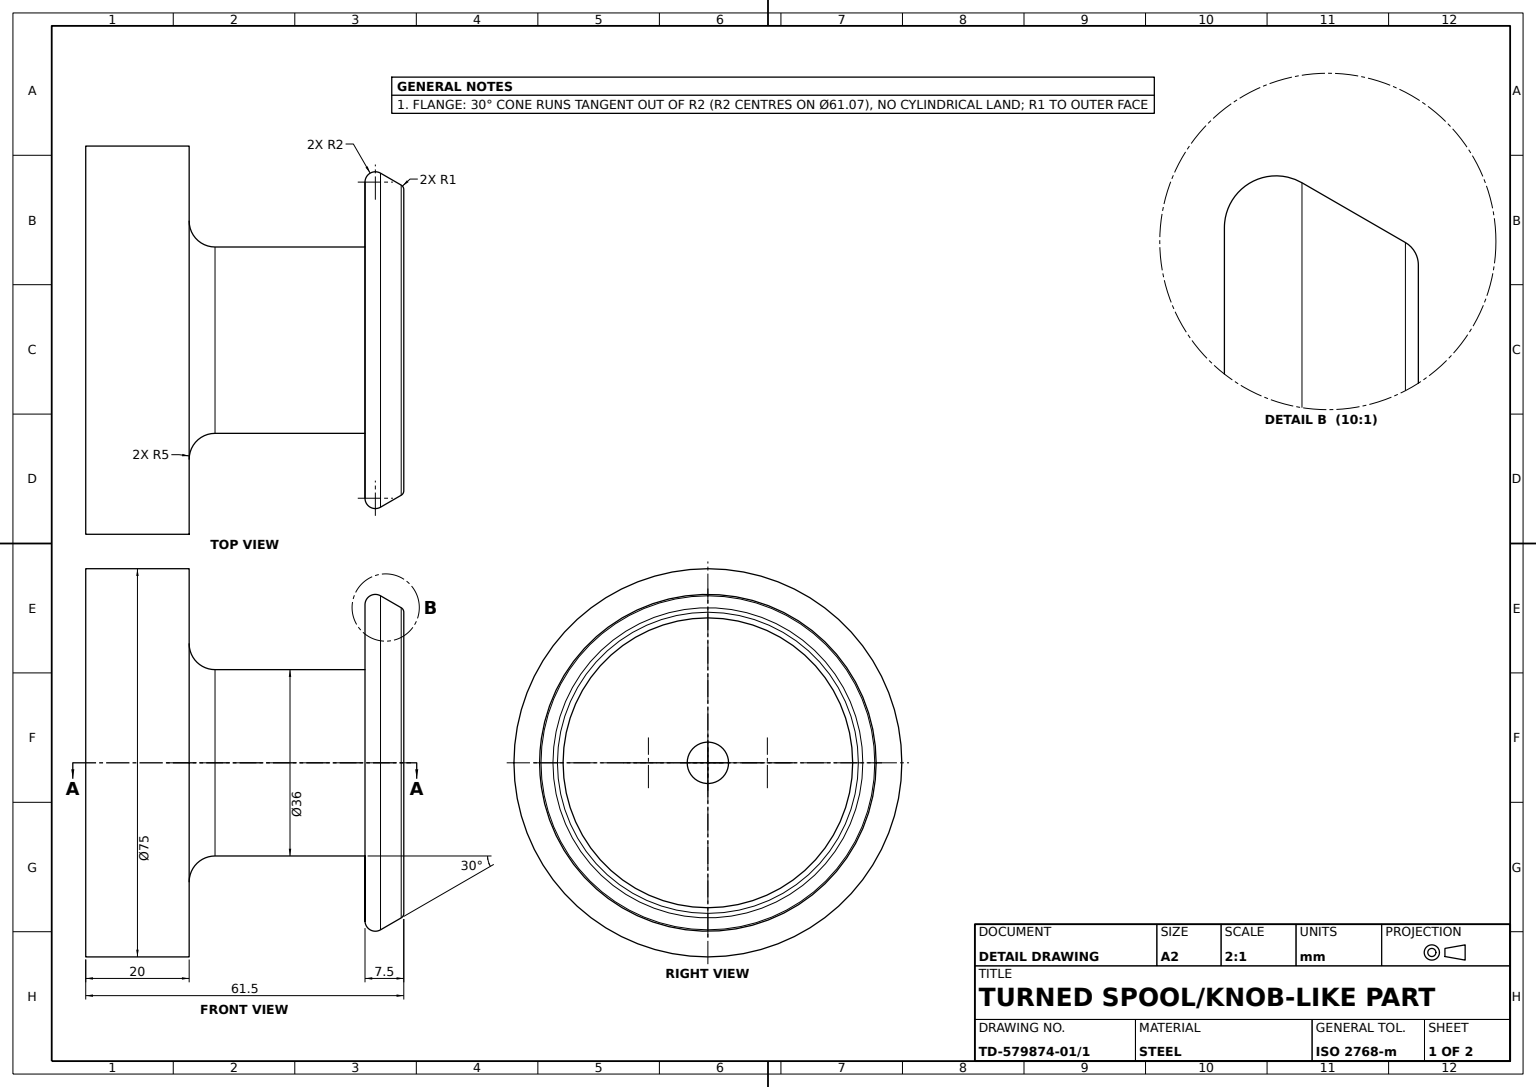
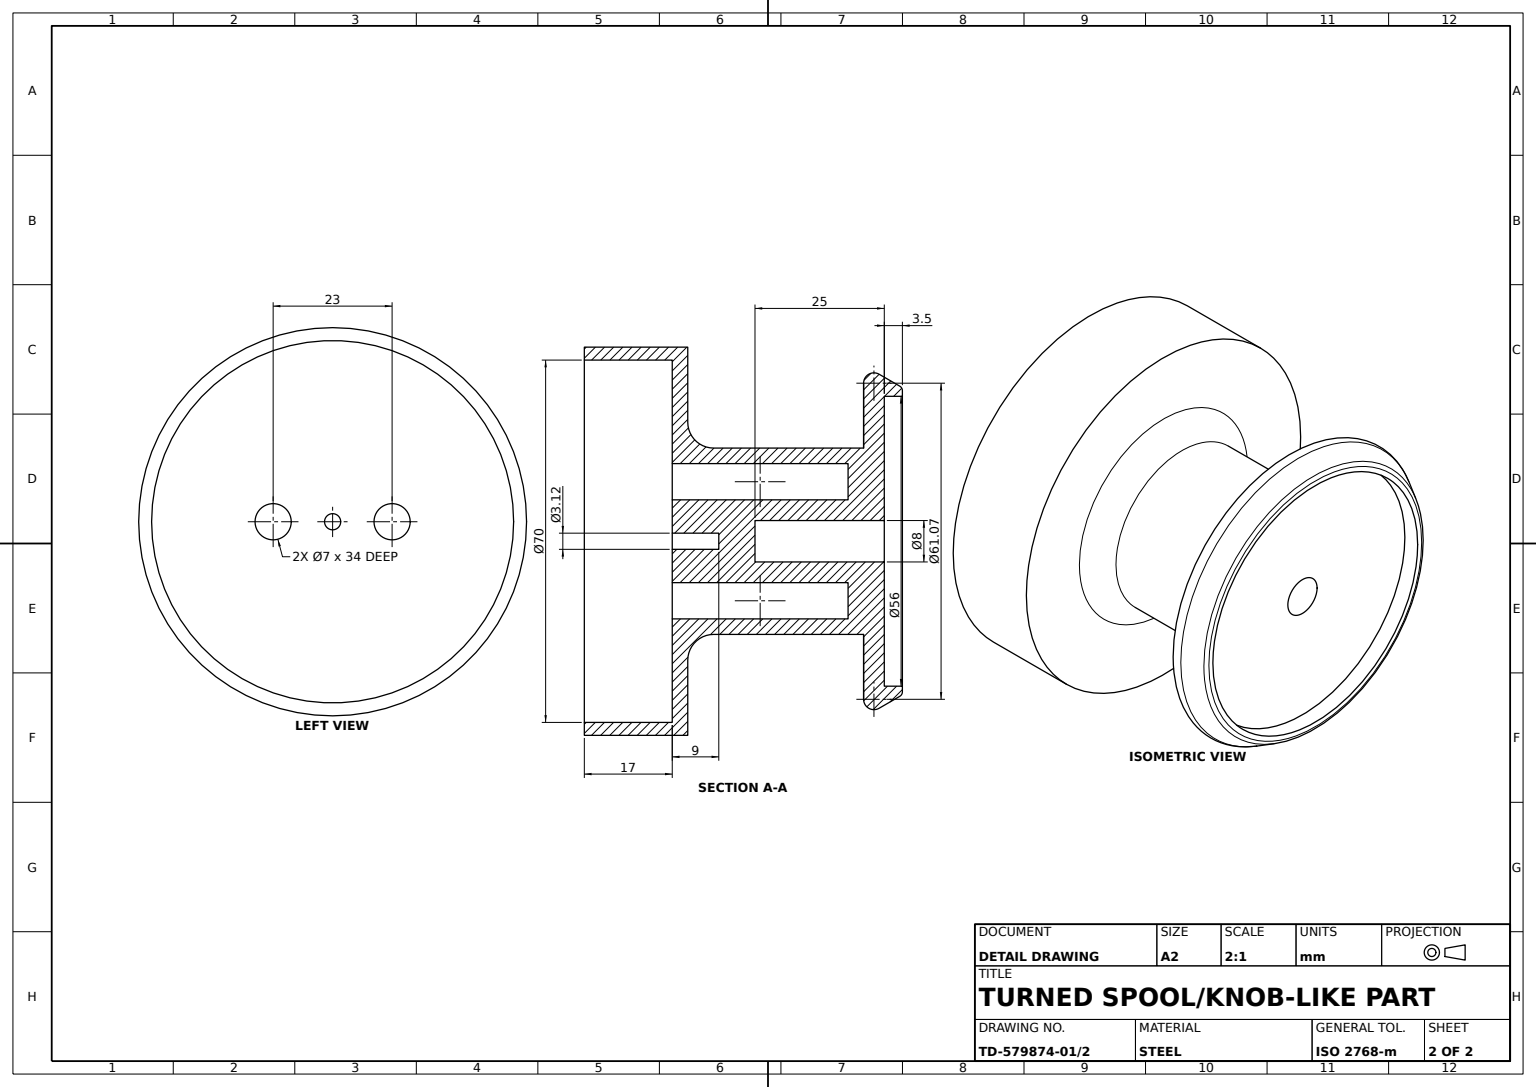
from build123d import *

# Parameters (mm, degrees)
BASE_DISC_SKETCH_75_R        = 37.5
BASE_DISC_75_DEPTH           = 20
NECK_SKETCH_36_R             = 18
NECK_36_DEPTH                = 34
NECK_ROOT_FILLET_R5_R        = 5
TOP_FLANGE_SKETCH_68_R       = 34
TOP_FLANGE_68_DRAFTED_DEPTH  = 7.5
TOP_FLANGE_68_DRAFTED_TAPER  = 30
TOP_RECESS_SKETCH_56_R       = 28
TOP_RECESS_56_DEPTH          = 3.5
FLANGE_EDGE_FILLET_R1_R      = 1
FLANGE_EDGE_FILLET_R2_R      = 2
BASE_RECESS_SKETCH_70_R      = 35
BASE_RECESS_70_DEPTH         = 17
BASE_POCKET_PROFILE_SKETCH_R = 3.5
BASE_POCKET_CUT_34MM_DEPTH   = 34
SKETCH32_4_R                 = 1.562112032
BASE_POCKET_CUT_9MM_DEPTH    = 9
CENTRE_HOLE_SKETCH_8_R       = 4
CENTRE_HOLE_8_DEPTH          = 25


with BuildPart() as part:
    # Base Disc Sketch _75 → Base Disc _75 (new body)
    with BuildSketch(Plane(origin=(0, 0, 0), x_dir=(1, 0, 0), z_dir=(0, 1, 0))):
        with Locations(Location((0, 0, 0), (0, 0, 270))):
            Circle(BASE_DISC_SKETCH_75_R)
    extrude(amount=BASE_DISC_75_DEPTH)

    # Neck Sketch _36 → Neck _36 (add)
    with BuildSketch(Plane(origin=(0, 20, 0), x_dir=(1, 0, 0), z_dir=(0, 1, 0))):
        with Locations(Location((0, 0, 0), (0, 0, 270))):
            Circle(NECK_SKETCH_36_R)
    extrude(amount=NECK_36_DEPTH)

    # Neck Root Fillet R5
    neck_root_fillet_r5_edges = [part.edges().sort_by_distance(p)[0] for p in [
        (0, 20, -18),
    ]]
    fillet(neck_root_fillet_r5_edges, radius=NECK_ROOT_FILLET_R5_R)

    # Top Flange Sketch _68 → Top Flange _68 Drafted (add)
    with BuildSketch(Plane(origin=(0, 54, 0), x_dir=(1, 0, 0), z_dir=(0, 1, 0))):
        Circle(TOP_FLANGE_SKETCH_68_R)
    extrude(amount=TOP_FLANGE_68_DRAFTED_DEPTH, taper=TOP_FLANGE_68_DRAFTED_TAPER)

    # Top Recess Sketch _56 → Top Recess _56 (cut)
    with BuildSketch(Plane(origin=(0, 61.5, 0), x_dir=(1, 0, 0), z_dir=(0, 1, 0))):
        with Locations(Location((0, 0, 0), (0, 0, 270))):
            Circle(TOP_RECESS_SKETCH_56_R)
    extrude(amount=-TOP_RECESS_56_DEPTH, mode=Mode.SUBTRACT)

    # Flange Edge Fillet R1
    flange_edge_fillet_r1_edges = [part.edges().sort_by_distance(p)[0] for p in [
        (-29.669872981, 61.5, 0),
    ]]
    fillet(flange_edge_fillet_r1_edges, radius=FLANGE_EDGE_FILLET_R1_R)

    # Flange Edge Fillet R2
    flange_edge_fillet_r2_edges = [part.edges().sort_by_distance(p)[0] for p in [
        (-34, 54, 0),
    ]]
    fillet(flange_edge_fillet_r2_edges, radius=FLANGE_EDGE_FILLET_R2_R)

    # Base Recess Sketch _70 → Base Recess _70 (cut)
    with BuildSketch(Plane.XZ):
        with Locations(Location((0, 0, 0), (0, 0, 270))):
            Circle(BASE_RECESS_SKETCH_70_R)
    extrude(amount=-BASE_RECESS_70_DEPTH, mode=Mode.SUBTRACT)

    # Base Pocket Profile Sketch → Base Pocket Cut 34mm (cut)
    with BuildSketch(Plane.XZ.offset(-17)):
        with Locations(Location((0, -11.5, 0), (0, 0, 270))):
            Circle(BASE_POCKET_PROFILE_SKETCH_R)
        with Locations(Location((0, 11.5, 0), (0, 0, 270))):
            Circle(BASE_POCKET_PROFILE_SKETCH_R)
    extrude(amount=-BASE_POCKET_CUT_34MM_DEPTH, mode=Mode.SUBTRACT)

    # Sketch32_4 → Base Pocket Cut 9mm (cut)
    with BuildSketch(Plane.XZ.offset(-17)):
        with Locations(Location((0, 0, 0), (0, 0, 270))):
            Circle(SKETCH32_4_R)
    extrude(amount=-BASE_POCKET_CUT_9MM_DEPTH, mode=Mode.SUBTRACT)

    # Centre Hole Sketch _8 → Centre Hole _8 (cut)
    with BuildSketch(Plane(origin=(0, 58, 0), x_dir=(1, 0, 0), z_dir=(0, 1, 0))):
        with Locations(Location((0, 0, 0), (0, 0, 270))):
            Circle(CENTRE_HOLE_SKETCH_8_R)
    extrude(amount=-CENTRE_HOLE_8_DEPTH, mode=Mode.SUBTRACT)


solid = part.part
